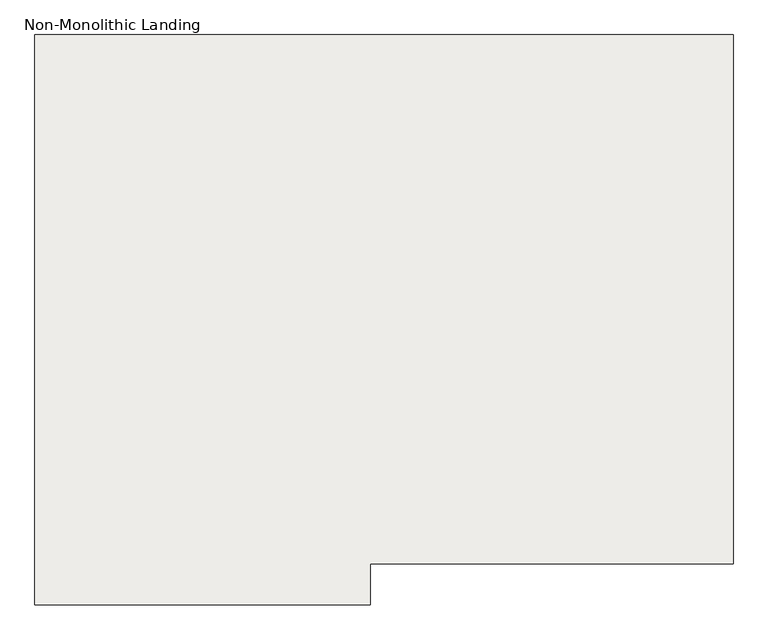
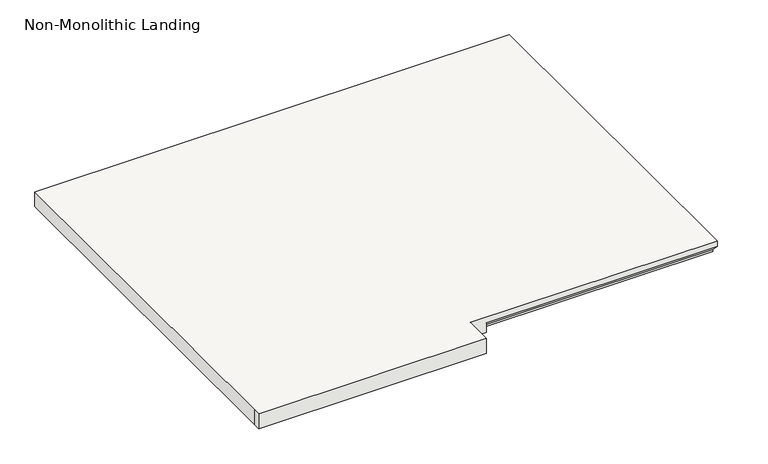
"""IFC4 building model written with IfcOpenShell, lengths in millimetres: slab geometry, Non-Monolithic Landing."""

from ifc_helpers import new_model, si_unit, origin, place, context, project, spatial, faceted_brep, source, transform, mapped, element, save


def non_monolithic_landing_99838e1e(model_context):
    return source(origin(), model_context, "Body", "Brep", [
        faceted_brep([(-5330.5155596, 6109.0076853, 4337.05), (-5330.5155596, 6083.6076853, 4362.45), (-6072.1955596, 6083.6076853, 4362.45), (-6072.1955596, 6109.0076853, 4337.05), (-5330.5155596, 7239.3076853, 4381.5), (-6854.5155596, 7239.3076853, 4381.5), (-6854.5155596, 6020.1076853, 4381.5), (-6854.5155596, 5994.7076853, 4381.5), (-6122.9955596, 5994.7076853, 4381.5), (-6122.9955596, 6020.1076853, 4381.5), (-6122.9955596, 6083.6076853, 4381.5), (-5330.5155596, 6083.6076853, 4381.5), (-6072.1955596, 6109.0076853, 4330.7), (-6072.1955596, 6083.6076853, 4330.7), (-6122.9955596, 6083.6076853, 4330.7), (-6122.9955596, 6020.1076853, 4330.7), (-6122.9955596, 5994.7076853, 4330.7), (-6854.5155596, 5994.7076853, 4330.7), (-6854.5155596, 6020.1076853, 4330.7), (-6854.5155596, 7239.3076853, 4330.7), (-5330.5155596, 7239.3076853, 4330.7), (-5330.5155596, 6109.0076853, 4330.7)], [[[0, 1, 2, 3]], [[4, 5, 6, 7, 8, 9, 10, 11]], [[12, 13, 14, 15, 16, 17, 18, 19, 20, 21]], [[13, 12, 3, 2]], [[12, 21, 0, 3]], [[4, 11, 1, 0, 21, 20]], [[5, 4, 20, 19]], [[6, 5, 19, 18]], [[7, 6, 18, 17]], [[8, 7, 17, 16]], [[9, 8, 16, 15]], [[10, 9, 15, 14]], [[11, 10, 14, 13, 2, 1]]]),
    ])


if __name__ == "__main__":
    model = new_model("IFC4")
    model_context = context("Model", 3, world=origin())
    ifc_project = project(units=[si_unit("LENGTHUNIT", "METRE", prefix="MILLI")], contexts=[model_context])
    site = spatial("IfcSite", under=ifc_project)
    building = spatial("IfcBuilding", under=site)
    placement = place(None, origin())
    non_monolithic_landing_shape = non_monolithic_landing_99838e1e(model_context)
    element("IfcSlab", 1, ObjectType="Non-Monolithic Landing", at=placement, inside=building, context=model_context, shape_type="MappedRepresentation", body=[
        mapped(non_monolithic_landing_shape, transform((0.0, 0.0, 0.0), x_axis=(1.0, 0.0, 0.0), y_axis=(0.0, 1.0, 0.0), z_axis=(0.0, 0.0, 1.0))),
    ])
    save(model, "model.ifc")
